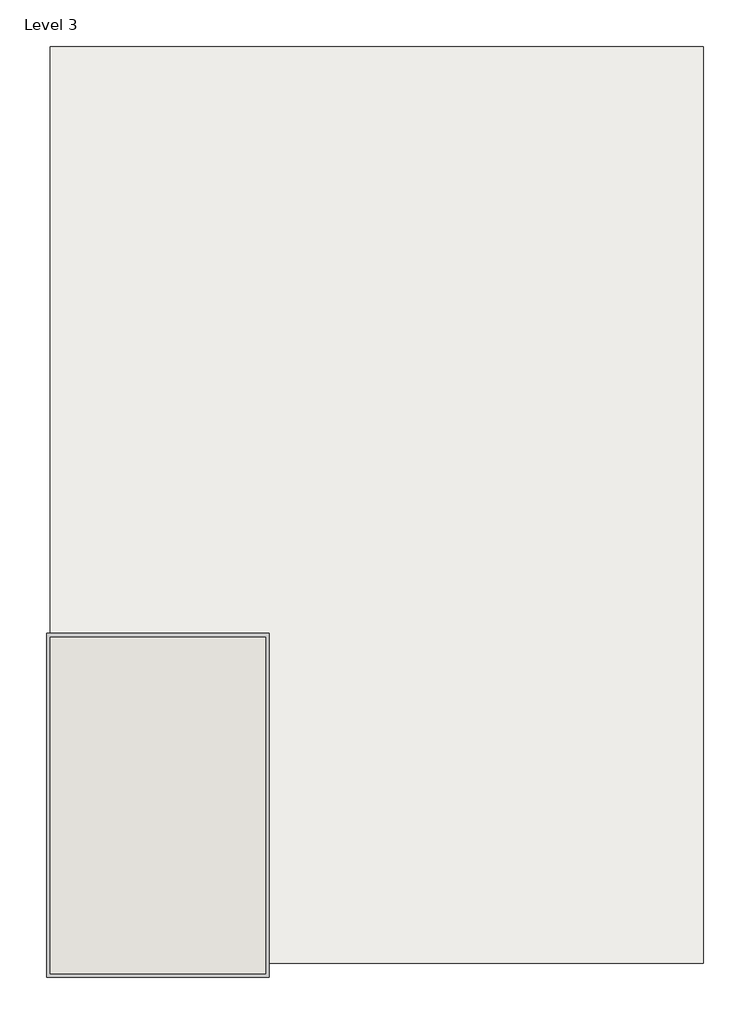
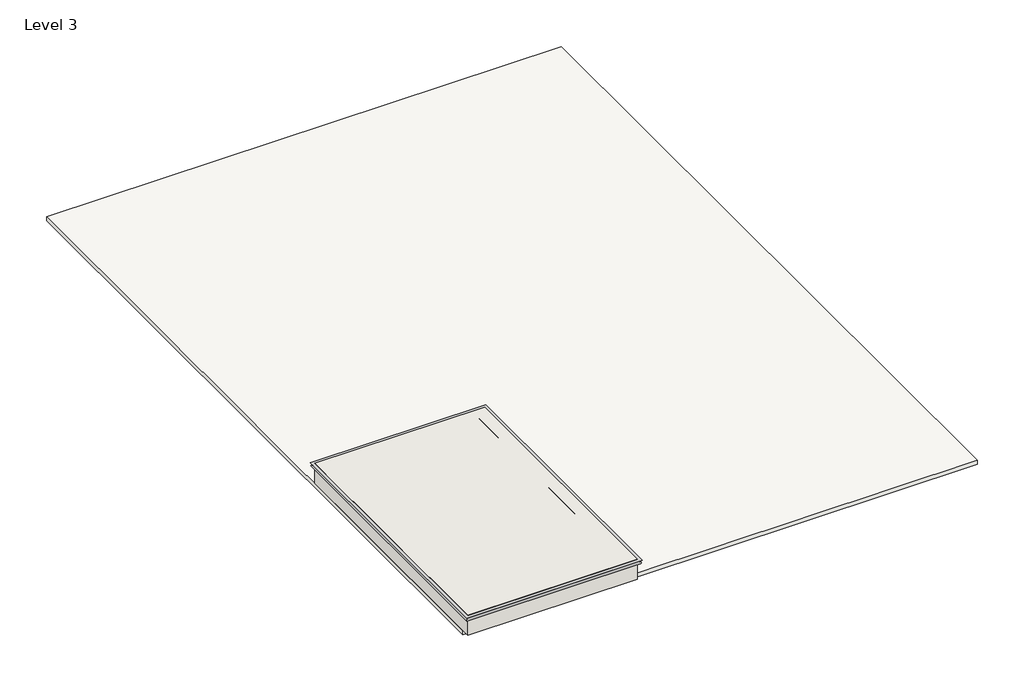
# One storey: 1 furniture element, 1 slab, 1 wall.
"""IFC4 building model written with IfcOpenShell, lengths in millimetres."""

from ifc_helpers import new_model, si_unit, frame, origin, place, context, project, spatial, polyline, outline, extrude, transform, mapped, element, save
from components import cs1_cs1_efe94d7d, walls_3_walls_3_115270fa

model = new_model("IFC4")

# Units and contexts
model_context = context("Model", 3, world=origin())
ifc_project = project(units=[si_unit("LENGTHUNIT", "METRE", prefix="MILLI")], contexts=[model_context])

# Site, building, storey
site = spatial("IfcSite", under=ifc_project)
building = spatial("IfcBuilding", under=site)
storey = spatial("IfcBuildingStorey", under=building, Name="Level 3", Elevation=6096.0)

# Furniture
placement = place(None, origin())
cs1_cs1_shape = cs1_cs1_efe94d7d(model_context)
element("IfcFurniture", 1, ObjectType="CS1 : CS1", at=placement, inside=storey, context=model_context, shape_type="MappedRepresentation", body=[
    mapped(cs1_cs1_shape, transform((0.0, 0.0, 0.0), x_axis=(1.0, 0.0, 0.0), y_axis=(0.0, 1.0, 0.0), z_axis=(0.0, 0.0, 1.0))),
])

# Slab
element("IfcSlab", 2, ObjectType="Generic 150mm", at=placement, inside=storey, context=model_context, shape_type="SweptSolid", body=[
    extrude(outline(polyline([(-8728.022521, 10061.9822151), (9759.977479, 10061.9822151), (9759.977479, -15855.5467593), (-8728.022521, -15855.5467593), (-8728.022521, 10061.9822151)])), frame((0.0, 0.0, 5943.6), z_axis=(0.0, 0.0, 1.0), x_axis=(1.0, 0.0, 0.0)), (0.0, 0.0, 1.0), 152.4),
])

# Wall
walls_3_walls_3_shape = walls_3_walls_3_115270fa(model_context)
element("IfcWall", 3, ObjectType="Walls 3 : Walls 3", at=placement, inside=storey, context=model_context, shape_type="MappedRepresentation", body=[
    mapped(walls_3_walls_3_shape, transform((0.0, 0.0, 0.0), x_axis=(1.0, 0.0, 0.0), y_axis=(0.0, 1.0, 0.0), z_axis=(0.0, 0.0, 1.0))),
])

save(model, "model.ifc")

# Revit data of these elements
# Type "Generic 150mm"
#   Function = 0
#   Layers, outside or top first: 152.4 mm no material (function 1)
# Element 1 (IfcFurniture, "CS1 : CS1")
#   Phase Created = New Construction
#   Materials on its faces: "Oak Flooring"
# Element 2 (IfcSlab, "Generic 150mm")
#   built-in parameter 1001955 = 3.14159 (stored number, unit not read)
#   Height Offset From Level = 0 mm
#   Phase Created = New Construction
#   Materials on its faces: "Default Floor", "CREAM WALL"
# Element 3 (IfcWall, "Walls 3 : Walls 3")
#   Phase Created = New Construction
#   Materials on its faces: "Default Wall"
# Materials
#   "Oak Flooring": class "Wood", colour RGB 212 179 113, transparency 0, Description = "Quercus Rubra", Cost = 0
#   "Default Floor": colour RGB 127 127 127, transparency 0
#   "CREAM WALL": colour RGB 255 255 187, transparency 0, Cost = 0
#   "Default Wall": colour RGB 128 128 128, transparency 0
